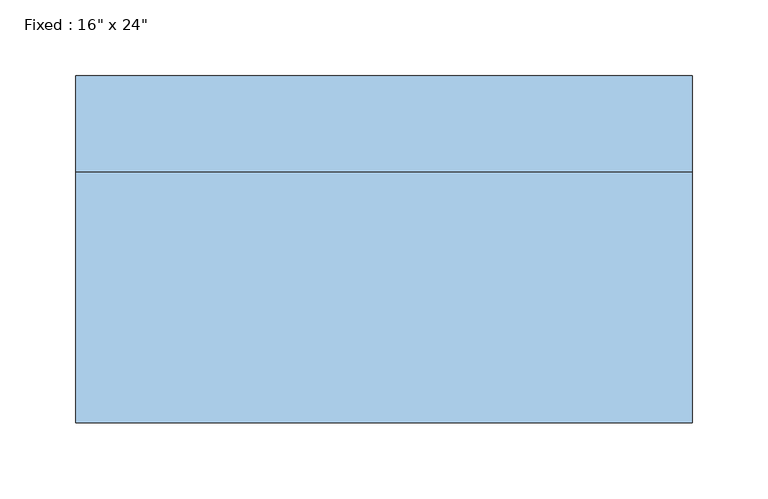
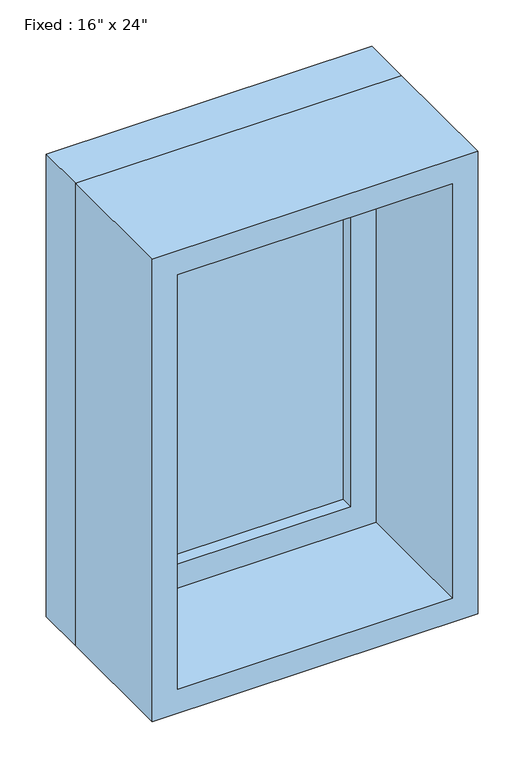
"""IFC4 building model written with IfcOpenShell, lengths in millimetres: window geometry."""

from ifc_helpers import new_model, si_unit, frame, origin, place, context, project, spatial, polyline, outline, extrude, source, transform, mapped, element, save


def window_aa618e30(model_context):
    return source(origin(), model_context, "Body", "SweptSolid", [
        extrude(outline(polyline([(101.6, 66.675), (-177.8, 66.675), (-177.8, 79.375), (101.6, 79.375), (101.6, 66.675)])), frame((0.0, 0.0, 977.9), z_axis=(0.0, 0.0, 1.0), x_axis=(1.0, 0.0, 0.0)), (0.0, 0.0, 1.0), 482.6),
        extrude(outline(polyline([(1504.95, -222.25), (933.45, -222.25), (933.45, 146.05), (1504.95, 146.05), (1504.95, -222.25)]), holes=[polyline([(1460.5, -177.8), (1460.5, 101.6), (977.9, 101.6), (977.9, -177.8), (1460.5, -177.8)])]), frame((0.0, 50.8, 0.0), z_axis=(0.0, 1.0, 0.0), x_axis=(0.0, 0.0, 1.0)), (0.0, 0.0, 1.0), 44.45),
        extrude(outline(polyline([(1524.0, -241.3), (914.4, -241.3), (914.4, 165.1), (1524.0, 165.1), (1524.0, -241.3)]), holes=[polyline([(1492.25, -209.55), (1492.25, 133.35), (946.15, 133.35), (946.15, -209.55), (1492.25, -209.55)])]), frame((0.0, -114.3, 0.0), z_axis=(0.0, 1.0, 0.0), x_axis=(0.0, 0.0, 1.0)), (0.0, 0.0, 1.0), 165.1),
        extrude(outline(polyline([(1524.0, 165.1), (1524.0, -241.3), (914.4, -241.3), (914.4, 165.1), (1524.0, 165.1)]), holes=[polyline([(1504.95, 146.05), (933.45, 146.05), (933.45, -222.25), (1504.95, -222.25), (1504.95, 146.05)])]), frame((0.0, 50.8, 0.0), z_axis=(0.0, 1.0, 0.0), x_axis=(0.0, 0.0, 1.0)), (0.0, 0.0, 1.0), 63.5),
    ])


if __name__ == "__main__":
    model = new_model("IFC4")
    model_context = context("Model", 3, world=origin())
    ifc_project = project(units=[si_unit("LENGTHUNIT", "METRE", prefix="MILLI")], contexts=[model_context])
    site = spatial("IfcSite", under=ifc_project)
    building = spatial("IfcBuilding", under=site)
    placement = place(None, origin())
    window_shape = window_aa618e30(model_context)
    element("IfcWindow", 1, ObjectType="Fixed : 16\" x 24\"", at=placement, inside=building, context=model_context, shape_type="MappedRepresentation", body=[
        mapped(window_shape, transform((0.0, 0.0, 0.0), x_axis=(1.0, 0.0, 0.0), y_axis=(0.0, 1.0, 0.0), z_axis=(0.0, 0.0, 1.0))),
    ])
    save(model, "model.ifc")

# Revit data of these elements
# Type "Fixed : 16\" x 24\""
#   Type Mark = "4"
#   Construction Type Id = "GSP4R"
#   Analytic Construction = "1/8 in Pilkington single glazing"
#   Visual Light Transmittance = 0.9
#   Solar Heat Gain Coefficient = 0.78
#   Heat Transfer Coefficient (U) = 0.6496 BTU/(h·ft²·°F)
#   Height = 2' - 0"
#   Default Sill Height = 3' - 0"
#   Width = 1' - 4"
#   Window Inset = 0' - 0 3/4"
#   Define Thermal Properties by = 1
#   Define Thermal Properties by = 1
#   Glass Pane Material = Glass
#   Sash Material = Sash
#   Wall Closure = (empty or 0)
# Element 1 (IfcWindow, "Fixed : 16\" x 24\"")
#   Materials on its faces: "Sash", "Glass"
# Materials
#   "Glass": class "Glass", colour RGB 0 128 192, transparency 0.75, Description = "Soda Lime Glass", Cost = 0
#   "Sash": class "Wood", colour RGB 224 178 126, transparency 0, Cost = 0
